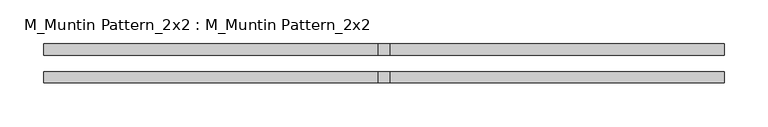
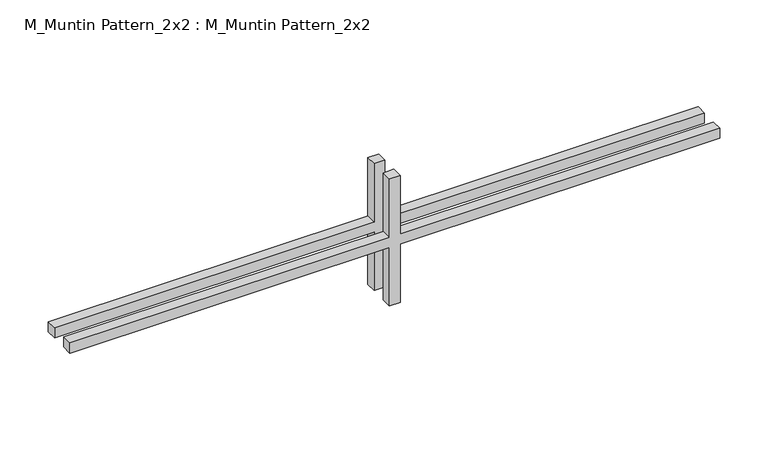
"""IFC4 building model written with IfcOpenShell, lengths in millimetres: proxy geometry, M_Muntin Pattern_2x2 : M_Muntin Pattern_2x2."""

from ifc_helpers import new_model, si_unit, frame, origin, place, context, project, spatial, polyline, outline, extrude, source, transform, mapped, element, save


def m_muntin_pattern_2x2_m_muntin_pattern_2x2_c118e93d(model_context):
    return source(origin(), model_context, "Body", "SweptSolid", [
        extrude(outline(polyline([(86.4955927, -6.35), (86.4955927, -387.35), (73.7955927, -387.35), (73.7955927, -6.35), (0.0, -6.35), (0.0, 6.35), (73.7955927, 6.35), (73.7955927, 387.35), (86.4955927, 387.35), (86.4955927, 6.35), (160.2911855, 6.35), (160.2911855, -6.35), (86.4955927, -6.35)])), frame((0.0, 9.525, 0.0), z_axis=(0.0, 1.0, 0.0), x_axis=(0.0, 0.0, 1.0)), (0.0, 0.0, 1.0), 12.7),
        extrude(outline(polyline([(86.4955927, -6.35), (86.4955927, -387.35), (73.7955927, -387.35), (73.7955927, -6.35), (0.0, -6.35), (0.0, 6.35), (73.7955927, 6.35), (73.7955927, 387.35), (86.4955927, 387.35), (86.4955927, 6.35), (160.2911855, 6.35), (160.2911855, -6.35), (86.4955927, -6.35)])), frame((0.0, -22.225, 0.0), z_axis=(0.0, 1.0, 0.0), x_axis=(0.0, 0.0, 1.0)), (0.0, 0.0, 1.0), 12.7),
    ])


if __name__ == "__main__":
    model = new_model("IFC4")
    model_context = context("Model", 3, world=origin())
    ifc_project = project(units=[si_unit("LENGTHUNIT", "METRE", prefix="MILLI")], contexts=[model_context])
    site = spatial("IfcSite", under=ifc_project)
    building = spatial("IfcBuilding", under=site)
    placement = place(None, origin())
    m_muntin_pattern_2x2_m_muntin_pattern_2x2_shape = m_muntin_pattern_2x2_m_muntin_pattern_2x2_c118e93d(model_context)
    element("IfcBuildingElementProxy", 1, Name="M_Muntin Pattern_2x2 : M_Muntin Pattern_2x2", ObjectType="M_Muntin Pattern_2x2 : M_Muntin Pattern_2x2", at=placement, inside=building, context=model_context, shape_type="MappedRepresentation", body=[
        mapped(m_muntin_pattern_2x2_m_muntin_pattern_2x2_shape, transform((0.0, 0.0, 0.0), x_axis=(1.0, 0.0, 0.0), y_axis=(0.0, 1.0, 0.0), z_axis=(0.0, 0.0, 1.0))),
    ])
    save(model, "model.ifc")

# Revit data of these elements
# Type "M_Muntin Pattern_2x2 : M_Muntin Pattern_2x2"
#   Width [instance default] = 3' - 11.24409"
#   Thickness = 0' - 0 1/2"
#   Height [instance default] = 3' - 11.24409"
#   Distance = 0' - 0 3/4"
#   Interior Material [instance default] = none
#   Exterior Material [instance default] = none
#   Default Elevation = 0
# Element 1 (IfcBuildingElementProxy, "M_Muntin Pattern_2x2 : M_Muntin Pattern_2x2")
#   Width = 2' - 6 1/2"
#   Height = 0' - 6.31068"
#   Interior Material = Wood - Stained
#   Exterior Material = Clad - White
#   Materials on its faces: "Clad - White", "Wood - Stained"
# Materials
#   "Clad - White": class "Wood", colour RGB 242 242 238, transparency 0, Cost = 0
#   "Wood - Stained": class "Wood", colour RGB 224 178 126, transparency 0, Cost = 0
